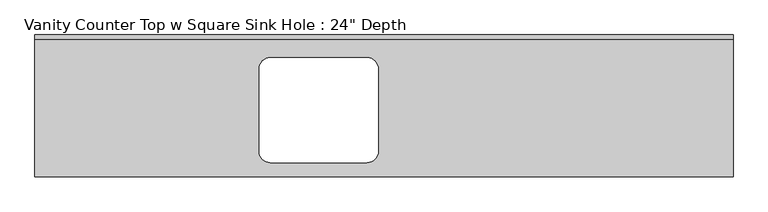
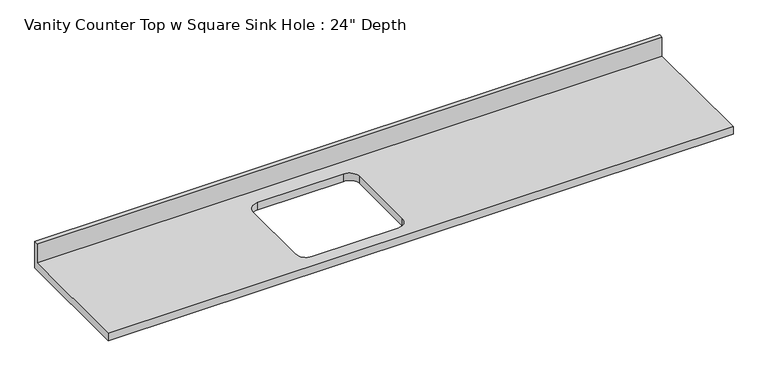
"""IFC4 building model written with IfcOpenShell, lengths in millimetres: furniture geometry."""

from ifc_helpers import new_model, si_unit, frame, origin, place, context, project, spatial, polyline, circle_curve, source, transform, mapped, element, save
from ifc_brep_helpers import plane_surface, revolved_surface, advanced_brep


def furniture_cbbb8910(model_context):
    return source(origin(), model_context, "Body", "AdvancedBrep", [
        advanced_brep(
        [(-1268.7247951, -635.0, 787.4), (1855.4836164, -635.0, 787.4), (1855.4836164, -19.05, 787.4), (-1268.7247951, -19.05, 787.4), (-265.4163836, -152.4, 787.4), (-214.6163836, -101.6, 787.4), (217.1836164, -101.6, 787.4), (267.9836164, -152.4, 787.4), (267.9836164, -520.7, 787.4), (217.1836164, -571.5, 787.4), (-214.6163836, -571.5, 787.4), (-265.4163836, -520.7, 787.4), (1855.4836164, 0.0, 749.3), (1855.4836164, -635.0, 749.3), (-1268.7247951, -635.0, 749.3), (-1268.7247951, 0.0, 749.3), (-214.6163836, -101.6, 749.3), (-265.4163836, -152.4, 749.3), (-265.4163836, -520.7, 749.3), (-214.6163836, -571.5, 749.3), (217.1836164, -571.5, 749.3), (267.9836164, -520.7, 749.3), (267.9836164, -152.4, 749.3), (217.1836164, -101.6, 749.3), (-1268.7247951, 0.0, 889.0), (1855.4836164, 0.0, 889.0), (-1268.7247951, -19.05, 889.0), (1855.4836164, -19.05, 889.0)],
        [
            (0, 1),
            (1, 2),
            (2, 3),
            (3, 0),
            (4, 5, circle_curve(frame((-214.6163836, -152.4, 787.4), z_axis=(0.0, 0.0, -1.0), x_axis=(1.0, 0.0, 0.0)), 50.8)),
            (5, 6),
            (6, 7, circle_curve(frame((217.1836164, -152.4, 787.4), z_axis=(0.0, 0.0, -1.0), x_axis=(1.0, 0.0, 0.0)), 50.8)),
            (7, 8),
            (8, 9, circle_curve(frame((217.1836164, -520.7, 787.4), z_axis=(0.0, 0.0, -1.0), x_axis=(1.0, 0.0, 0.0)), 50.8)),
            (9, 10),
            (10, 11, circle_curve(frame((-214.6163836, -520.7, 787.4), z_axis=(0.0, 0.0, -1.0), x_axis=(1.0, 0.0, 0.0)), 50.8)),
            (11, 4),
            (12, 13),
            (13, 14),
            (14, 15),
            (15, 12),
            (16, 17, circle_curve(frame((-214.6163836, -152.4, 749.3), z_axis=(0.0, 0.0, 1.0), x_axis=(1.0, 0.0, 0.0)), 50.8)),
            (17, 18),
            (18, 19, circle_curve(frame((-214.6163836, -520.7, 749.3), z_axis=(0.0, 0.0, 1.0), x_axis=(1.0, 0.0, 0.0)), 50.8)),
            (19, 20),
            (20, 21, circle_curve(frame((217.1836164, -520.7, 749.3), z_axis=(0.0, 0.0, 1.0), x_axis=(1.0, 0.0, 0.0)), 50.8)),
            (21, 22),
            (22, 23, circle_curve(frame((217.1836164, -152.4, 749.3), z_axis=(0.0, 0.0, 1.0), x_axis=(1.0, 0.0, 0.0)), 50.8)),
            (23, 16),
            (15, 24),
            (24, 25),
            (25, 12),
            (14, 0),
            (3, 26),
            (26, 24),
            (13, 1),
            (25, 27),
            (27, 2),
            (26, 27),
            (4, 17),
            (16, 5),
            (11, 18),
            (10, 19),
            (9, 20),
            (8, 21),
            (7, 22),
            (6, 23),
        ],
        [
            plane_surface(frame((-1268.7247951, 0.0, 787.4), z_axis=(0.0, 0.0, 1.0), x_axis=(-1.0, 0.0, 0.0))),
            plane_surface(frame((-1268.7247951, 0.0, 749.3), z_axis=(0.0, 0.0, -1.0), x_axis=(1.0, 0.0, 0.0))),
            plane_surface(frame((1855.4836164, 0.0, 787.4), z_axis=(0.0, 1.0, 0.0), x_axis=(0.0, 0.0, -1.0))),
            plane_surface(frame((-1268.7247951, 0.0, 787.4), z_axis=(-1.0, 0.0, 0.0), x_axis=(0.0, 0.0, -1.0))),
            plane_surface(frame((-1268.7247951, -635.0, 787.4), z_axis=(0.0, -1.0, 0.0), x_axis=(0.0, 0.0, -1.0))),
            plane_surface(frame((1855.4836164, -635.0, 787.4), z_axis=(1.0, 0.0, 0.0), x_axis=(0.0, 0.0, -1.0))),
            plane_surface(frame((-1268.7247951, 0.0, 889.0), z_axis=(0.0, 0.0, 1.0), x_axis=(0.0, -1.0, 0.0))),
            plane_surface(frame((-1268.7247951, -19.05, 889.0), z_axis=(0.0, -1.0, 0.0), x_axis=(0.0, 0.0, -1.0))),
            revolved_surface(polyline([(-163.8163836, -152.4, 787.4), (-163.8163836, -152.4, 749.3)]), (-214.6163836, -152.4, 749.3), (0.0, 0.0, 1.0)),
            plane_surface(frame((-265.4163836, -152.4, 787.4), z_axis=(1.0, 0.0, 0.0), x_axis=(0.0, 0.0, -1.0))),
            revolved_surface(polyline([(-163.8163836, -520.7, 787.4), (-163.8163836, -520.7, 749.3)]), (-214.6163836, -520.7, 749.3), (0.0, 0.0, 1.0)),
            plane_surface(frame((-214.6163836, -571.5, 787.4), z_axis=(0.0, 1.0, 0.0), x_axis=(0.0, 0.0, -1.0))),
            revolved_surface(polyline([(267.9836164, -520.7, 787.4), (267.9836164, -520.7, 749.3)]), (217.1836164, -520.7, 749.3), (0.0, 0.0, 1.0)),
            plane_surface(frame((267.9836164, -520.7, 787.4), z_axis=(-1.0, 0.0, 0.0), x_axis=(0.0, 0.0, -1.0))),
            revolved_surface(polyline([(267.9836164, -152.4, 787.4), (267.9836164, -152.4, 749.3)]), (217.1836164, -152.4, 749.3), (0.0, 0.0, 1.0)),
            plane_surface(frame((217.1836164, -101.6, 787.4), z_axis=(0.0, -1.0, 0.0), x_axis=(0.0, 0.0, -1.0))),
        ],
        [
            (0, [[1, 2, 3, 4], [5, 6, 7, 8, 9, 10, 11, 12]]),
            (1, [[13, 14, 15, 16], [17, 18, 19, 20, 21, 22, 23, 24]]),
            (2, [[-16, 25, 26, 27]]),
            (3, [[-15, 28, -4, 29, 30, -25]]),
            (4, [[-1, -28, -14, 31]]),
            (5, [[-13, -27, 32, 33, -2, -31]]),
            (6, [[-30, 34, -32, -26]]),
            (7, [[-34, -29, -3, -33]]),
            (8, [[35, -17, 36, -5]]),
            (9, [[-35, -12, 37, -18]]),
            (10, [[-37, -11, 38, -19]]),
            (11, [[-38, -10, 39, -20]]),
            (12, [[-39, -9, 40, -21]]),
            (13, [[-40, -8, 41, -22]]),
            (14, [[-41, -7, 42, -23]]),
            (15, [[-36, -24, -42, -6]]),
        ],
    ),
    ])


if __name__ == "__main__":
    model = new_model("IFC4")
    model_context = context("Model", 3, world=origin())
    ifc_project = project(units=[si_unit("LENGTHUNIT", "METRE", prefix="MILLI")], contexts=[model_context])
    site = spatial("IfcSite", under=ifc_project)
    building = spatial("IfcBuilding", under=site)
    placement = place(None, origin())
    furniture_shape = furniture_cbbb8910(model_context)
    element("IfcFurniture", 1, ObjectType="Vanity Counter Top w Square Sink Hole : 24\" Depth", at=placement, inside=building, context=model_context, shape_type="MappedRepresentation", body=[
        mapped(furniture_shape, transform((0.0, 0.0, 0.0), x_axis=(1.0, 0.0, 0.0), y_axis=(0.0, 1.0, 0.0), z_axis=(0.0, 0.0, 1.0))),
    ])
    save(model, "model.ifc")

# Revit data of these elements
# Type "Vanity Counter Top w Square Sink Hole : 24\" Depth"
#   Assembly Code = "C1030400"
#   Counter Thickness = 0' - 1 1/2"
#   Depth = 2' - 1"
#   Height = 2' - 7"
#   Length [instance default] = 4' - 0"
#   Sink Location [instance default] = 2' - 0"
#   Sink Location To Wall [instance default] = 0' - 4 1/2"
#   Sink Opening Depth [instance default] = 1' - 5 1/2"
#   Sink Opening Width [instance default] = 1' - 8"
#   Counter Top Material = none
#   Default Elevation = 0
# Element 1 (IfcFurniture, "Vanity Counter Top w Square Sink Hole : 24\" Depth")
#   Length = 10' - 3.00033"
#   Sink Location = 4' - 2.00033"
#   Materials on its faces: "Counter Top"
# Materials
#   "Counter Top": class "Wood", colour RGB 226 177 128, transparency 0
